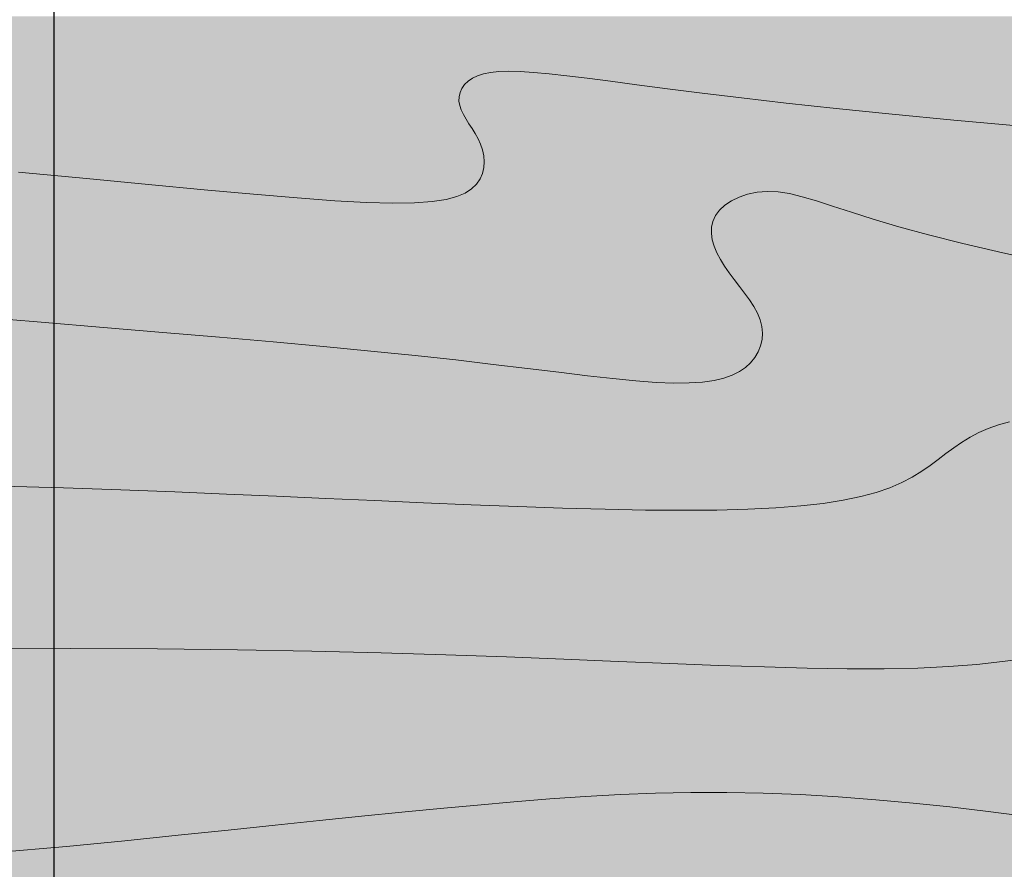
# Model space of a CAD drawing. Units: inches. Extents: x 2549 to 3108, y 1683 to 2362.
# Tile 12 of 30: x 2734 to 2749, y 2028 to 2041. Entities that reach past the tile are written whole.
import ezdxf

# ---------------------------------------------------------------- set-up
doc = ezdxf.new("R2010")
doc.units = ezdxf.units.IN
for name, color, linetype, lineweight in [('A-ANNO-DIMS', 2, 'Continuous', 18), ('A-FURN', 8, 'Continuous', 18), ('A-FURN-PATT', 9, 'Continuous', 13)]:
    doc.layers.add(name, color=color, linetype=linetype, lineweight=lineweight)
doc.layers.add('C-PKNG-VEHI-PATT', color=251, linetype='Continuous', lineweight=13, true_color=0x636466)
doc.layers.add('C-PVMT-PATT', color=9, linetype='Continuous', lineweight=13, true_color=0xc7c8ca)
doc.styles.get("Standard").update_dxf_attribs({"font": 'arial.ttf'})
doc.dimstyles.get("Standard").update_dxf_attribs({"dimtxt": 0.18, "dimasz": 0.18, "dimexe": 0.18, "dimexo": 0.0625, "dimgap": 0.09, "dimtad": 0, "dimtih": 1, "dimtoh": 1, "dimdec": 4, "dimzin": 0, "dimdsep": 46, "dimtxsty": 'Standard', "dimcen": 0.09, "dimadec": 0, "dimazin": 0, "dimtfac": 1, "dimtdec": 4, "dimtofl": 0, "dimtmove": 0, "dimatfit": 3, "dimfxl": 1, "dimtolj": 1, "dimtzin": 0, "dimarcsym": 0})

# ---------------------------------------------------------------- blocks, each defined once
blk = doc.blocks.new('Dining Set - 36 x 72 in.')
for points in [[(-3.6035, 13.63021), (-1.6954, 13.45508), (0.0365, 13.29166), (1.5945, 13.14388), (2.9811, 13.01562), (4.1988, 12.9108), (5.25, 12.83333), (6.1393, 12.78613), (6.8802, 12.76823), (7.4883, 12.77767), (7.9792, 12.8125), (8.3685, 12.87077), (8.6719, 12.95052), (8.9049, 13.0498), (9.0833, 13.16666), (9.2205, 13.29899), (9.3216, 13.44401), (9.3895, 13.59879), (9.4271, 13.76041), (9.4373, 13.92594), (9.4232, 14.09245), (9.3875, 14.257), (9.3333, 14.41666), (9.2638, 14.56917), (9.1836, 14.71484), (9.0975, 14.85465), (9.0104, 14.98958), (8.9272, 15.1206), (8.8529, 15.2487), (8.7922, 15.37483), (8.75, 15.5), (8.7305, 15.62467), (8.7344, 15.74739), (8.7617, 15.86621), (8.8125, 15.97916), (8.8867, 16.08431), (8.9844, 16.17968), (9.1055, 16.26334), (9.25, 16.33333), (9.4189, 16.38802), (9.6172, 16.42708), (9.8506, 16.45052), (10.125, 16.45833), (10.4463, 16.45052), (10.8203, 16.42708), (11.2529, 16.38802), (11.75, 16.33333), (12.3184, 16.26318), (12.9694, 16.17838), (13.7151, 16.07991), (14.5677, 15.96875), (15.5395, 15.84586), (16.6426, 15.71224), (17.8893, 15.56884), (19.2917, 15.41666), (20.859, 15.25667), (22.5879, 15.08984), (24.4721, 14.91715)], [(-4.7917, 9.58333), (-2.9698, 9.43082), (-1.2246, 9.28515), (0.4415, 9.14534), (2.026, 9.01041), (3.5266, 8.87939), (4.9408, 8.7513), (6.266, 8.62516), (7.5, 8.5), (8.6411, 8.37549), (9.6914, 8.2539), (10.6538, 8.13818), (11.5312, 8.03125), (12.3267, 7.93603), (13.043, 7.85547), (13.6831, 7.79248), (14.25, 7.75), (14.7471, 7.7303), (15.1797, 7.73307), (15.5537, 7.75732), (15.875, 7.80208), (16.1494, 7.86637), (16.3828, 7.94922), (16.5811, 8.04964), (16.75, 8.16666), (16.8944, 8.29915), (17.0143, 8.44531), (17.1089, 8.60319), (17.1771, 8.77083), (17.218, 8.94629), (17.2305, 9.1276), (17.2137, 9.31282), (17.1667, 9.5), (17.0895, 9.6875), (16.987, 9.875), (16.8649, 10.0625), (16.7292, 10.25), (16.5856, 10.4375), (16.4401, 10.625), (16.2985, 10.8125), (16.1667, 11), (16.05, 11.18733), (15.9518, 11.3737), (15.8752, 11.5581), (15.8229, 11.73958), (15.798, 11.91715), (15.8034, 12.08984), (15.842, 12.25667), (15.9167, 12.41666), (16.0295, 12.56836), (16.1784, 12.70833), (16.3605, 12.83268), (16.5729, 12.9375), (16.8127, 13.01888), (17.0768, 13.07291), (17.3625, 13.0957), (17.6667, 13.08333), (17.9894, 13.03312), (18.3418, 12.94726), (18.7382, 12.82918), (19.1927, 12.68229), (19.7195, 12.51001), (20.3327, 12.31575), (21.0465, 12.10294), (21.875, 11.875), (22.8357, 11.63354), (23.959, 11.37304), (25.2786, 11.08618)], [(-4.0586, 4.83984), (-2.3429, 4.79215), (-0.7396, 4.73958), (0.7739, 4.6831), (2.22, 4.6237), (3.6213, 4.56233), (5, 4.5), (6.373, 4.43782), (7.7344, 4.3776), (9.0723, 4.32129), (10.375, 4.27083), (11.6309, 4.22819), (12.8281, 4.19531), (13.9551, 4.17415), (15, 4.16666), (15.954, 4.17448), (16.819, 4.19791), (17.6001, 4.23698), (18.3021, 4.29166), (18.9299, 4.36198), (19.4883, 4.44791), (19.9823, 4.54948), (20.4167, 4.66666), (20.7969, 4.79899), (21.1302, 4.94401), (21.4245, 5.09879), (21.6875, 5.26041), (21.9271, 5.42594), (22.1511, 5.59245), (22.3672, 5.757), (22.5834, 5.91666), (22.8065, 6.06868), (23.0404, 6.21093), (23.2879, 6.34147), (23.5521, 6.45833), (23.8358, 6.55957), (24.142, 6.64323)], [(-4.75, 0.29166), (-2.134, 0.29793), (0.2878, 0.28711), (2.5317, 0.26163), (4.6146, 0.22396), (6.5529, 0.17651), (8.3633, 0.12174), (10.0623, 0.06209), (11.6667, 0), (13.1899, -0.06201), (14.6341, -0.1211), (15.9982, -0.17432), (17.2813, -0.21875), (18.4823, -0.25147), (19.6003, -0.26953), (20.6343, -0.27002), (21.5834, -0.25), (22.4481, -0.20768), (23.2357, -0.14584), (23.9549, -0.06836), (24.6146, 0.02083)], [(-4.2363, -5.41016), (-2.2629, -5.24333), (-0.625, -5.08334), (0.8708, -4.93099), (2.2715, -4.78646), (3.5872, -4.64974), (4.8281, -4.52084), (6.0046, -4.39974), (7.127, -4.28646), (8.2053, -4.18099), (9.25, -4.08334), (10.2705, -3.99382), (11.2734, -3.91407), (12.2647, -3.84603), (13.25, -3.79167), (14.2354, -3.75293), (15.2266, -3.73177), (16.2295, -3.73015), (17.25, -3.75), (18.2912, -3.79248), (19.3451, -3.85547), (20.4009, -3.93604), (21.4479, -4.03125), (22.4754, -4.13819), (23.4727, -4.25391), (24.4289, -4.37549)]]:
    blk.add_lwpolyline(points)
blk = doc.blocks.new('*D43')
at = {"layer": 'A-ANNO-DIMS', "color": 0, "lineweight": -2, "transparency": 16777216}
for p, q in [((2734.643, 2080.461), (2734.643, 1683.444)), ((2806.643, 2080.461), (2806.643, 1683.444)), ((2734.823, 1683.624), (2770.425, 1683.624)), ((2806.463, 1683.624), (2770.86, 1683.624))]:
    blk.add_line(p, q, dxfattribs=at)
at = {"layer": 'A-ANNO-DIMS', "color": 0, "transparency": 16777216}
for points in [[(2734.823, 1683.654), (2734.823, 1683.594), (2734.643, 1683.624)], [(2806.463, 1683.654), (2806.463, 1683.594), (2806.643, 1683.624)]]:
    blk.add_solid(points, dxfattribs=at)
at = {"layer": 'Defpoints', "color": 0, "transparency": 16777216}
for p in [(2734.643, 2080.524), (2806.643, 2080.524), (2806.643, 1683.624)]:
    blk.add_point(p, dxfattribs=at)
at = {"layer": 'A-ANNO-DIMS', "color": 0, "transparency": 16777216, "insert": (2770.643, 1683.624), "char_height": 0.18, "attachment_point": 5}
blk.add_mtext('\\A1;72', dxfattribs=at)
blk = doc.blocks.new('*D44')
at = {"layer": 'A-ANNO-DIMS', "color": 0, "lineweight": -2, "transparency": 16777216}
for p, q in [((2662.643, 2040.993), (2662.643, 1683.444)), ((2806.643, 2016.129), (2806.643, 1683.444)), ((2662.823, 1683.624), (2734.363, 1683.624)), ((2806.463, 1683.624), (2734.923, 1683.624))]:
    blk.add_line(p, q, dxfattribs=at)
at = {"layer": 'A-ANNO-DIMS', "color": 0, "transparency": 16777216}
for points in [[(2662.823, 1683.654), (2662.823, 1683.594), (2662.643, 1683.624)], [(2806.463, 1683.654), (2806.463, 1683.594), (2806.643, 1683.624)]]:
    blk.add_solid(points, dxfattribs=at)
at = {"layer": 'Defpoints', "color": 0, "transparency": 16777216}
for p in [(2662.643, 2041.056), (2806.643, 2016.191), (2806.643, 1683.624)]:
    blk.add_point(p, dxfattribs=at)
at = {"layer": 'A-ANNO-DIMS', "color": 0, "transparency": 16777216, "insert": (2734.643, 1683.624), "char_height": 0.18, "attachment_point": 5}
blk.add_mtext('\\A1;144', dxfattribs=at)
blk = doc.blocks.new('*D59')
at = {"layer": 'A-ANNO-DIMS', "color": 0, "lineweight": -2, "transparency": 16777216}
for p, q in [((2680.978, 1761.586), (2680.978, 2362.323)), ((2786.158, 1761.586), (2786.158, 2362.323)), ((2681.158, 2362.143), (2733.112, 2362.143)), ((2785.978, 2362.143), (2734.023, 2362.143))]:
    blk.add_line(p, q, dxfattribs=at)
at = {"layer": 'A-ANNO-DIMS', "color": 0, "transparency": 16777216}
for points in [[(2681.158, 2362.173), (2681.158, 2362.113), (2680.978, 2362.143)], [(2785.978, 2362.173), (2785.978, 2362.113), (2786.158, 2362.143)]]:
    blk.add_solid(points, dxfattribs=at)
at = {"layer": 'Defpoints', "color": 0, "transparency": 16777216}
for p in [(2786.158, 2362.143), (2680.978, 1761.524), (2786.158, 1761.524)]:
    blk.add_point(p, dxfattribs=at)
at = {"layer": 'A-ANNO-DIMS', "color": 0, "transparency": 16777216, "insert": (2733.568, 2362.143), "char_height": 0.18, "attachment_point": 5}
blk.add_mtext('\\A1;105.18', dxfattribs=at)

msp = doc.modelspace()

# ---------------------------------------------------------------- hatches: boundary and pattern name
at = {"layer": 'A-FURN-PATT'}
h = msp.add_hatch(color=256, dxfattribs=at)
h.dxf.hatch_style = 1
h.paths.add_polyline_path([(2744.8667, 2037.254), (2744.7754, 2037.3839), (2744.7125, 2037.4849), (2744.6595, 2037.5854), (2744.5963, 2037.7375), (2744.5695, 2037.9287), (2744.6003, 2038.0617), (2744.6406, 2038.148), (2744.7014, 2038.2298), (2744.7817, 2038.3053), (2744.8799, 2038.3724), (2744.9945, 2038.4289), (2745.1238, 2038.4728), (2745.2663, 2038.5019), (2745.4204, 2038.5142), (2745.5844, 2038.5076), (2745.7585, 2038.4805), (2745.9486, 2038.4342), (2746.1624, 2038.3705), (2746.4075, 2038.2913), (2746.6917, 2038.1983), (2747.0224, 2038.0936), (2747.4074, 2037.9788), (2747.8543, 2037.8558), (2748.3724, 2037.7256), (2748.9783, 2037.5851), (2749.69, 2037.4304), (2750.5258, 2037.2575), (2751.5038, 2037.0624), (2752.6422, 2036.8414), (2753.9591, 2036.5902), (2755.4728, 2036.3051), (2755.4728, 2039.002), (2754.0892, 2039.103), (2752.7721, 2039.2035), (2751.5251, 2039.303), (2750.3516, 2039.4009), (2749.255, 2039.4967), (2748.2388, 2039.5898), (2747.3063, 2039.6798), (2746.4609, 2039.7661), (2745.7045, 2039.8482), (2745.0321, 2039.9255), (2744.4371, 2039.9976), (2743.9129, 2040.0639), (2743.4531, 2040.1238), (2743.0509, 2040.1769), (2742.6998, 2040.2227), (2742.3932, 2040.2605), (2742.1251, 2040.29), (2741.8917, 2040.3111), (2741.69, 2040.3237), (2741.5167, 2040.3279), (2741.3687, 2040.3237), (2741.2428, 2040.3111), (2741.1359, 2040.29), (2741.0448, 2040.2605), (2740.9668, 2040.2227), (2740.9015, 2040.1776), (2740.8488, 2040.1262), (2740.8088, 2040.0695), (2740.7814, 2040.0085), (2740.7667, 2039.9445), (2740.7646, 2039.8783), (2740.7751, 2039.811), (2740.7978, 2039.7435), (2740.8306, 2039.6755), (2740.8707, 2039.6064), (2740.9155, 2039.5357), (2740.996, 2039.4111), (2741.0771, 2039.2637), (2741.1346, 2039.0945), (2741.1499, 2038.9139), (2741.1092, 2038.7391), (2741.0289, 2038.6239), (2740.9549, 2038.5525), (2740.8586, 2038.4895), (2740.733, 2038.4359), (2740.5693, 2038.3929), (2740.3593, 2038.3615), (2740.0946, 2038.3427), (2739.7666, 2038.3376), (2739.367, 2038.3473), (2738.8873, 2038.3727), (2738.3203, 2038.4145), (2737.6635, 2038.471), (2736.9156, 2038.5402), (2736.0753, 2038.6199), (2735.1412, 2038.7081), (2734.112, 2038.8025), (2732.9864, 2038.9012), (2731.7632, 2039.002), (2730.4376, 2039.1026), (2728.9922, 2039.2), (2727.4062, 2039.2911), (2725.6588, 2039.3728), (2723.7291, 2039.4418), (2721.5964, 2039.495), (2719.2397, 2039.5292), (2716.6384, 2039.5413), (2716.6384, 2036.8445), (2720.4266, 2036.9215), (2723.5572, 2036.9548), (2726.1183, 2036.9512), (2728.1983, 2036.9175), (2729.8853, 2036.8608), (2731.2677, 2036.7876), (2732.4336, 2036.705), (2733.4711, 2036.6198), (2734.4538, 2036.5375), (2735.3951, 2036.4589), (2736.2938, 2036.3835), (2737.1484, 2036.3108), (2737.9578, 2036.2401), (2738.7205, 2036.171), (2739.4353, 2036.103), (2740.1009, 2036.0355), (2740.7163, 2035.9683), (2741.2828, 2035.9027), (2741.8019, 2035.8403), (2742.2752, 2035.7826), (2742.7042, 2035.7313), (2743.0906, 2035.6878), (2743.4358, 2035.6539), (2743.7416, 2035.6309), (2744.0097, 2035.6203), (2744.243, 2035.6218), (2744.4448, 2035.6349), (2744.6181, 2035.659), (2744.7661, 2035.6937), (2744.892, 2035.7384), (2744.9989, 2035.7926), (2745.09, 2035.8557), (2745.1679, 2035.9271), (2745.2326, 2036.006), (2745.2836, 2036.0911), (2745.3204, 2036.1815), (2745.3424, 2036.2762), (2745.3492, 2036.374), (2745.3401, 2036.4739), (2745.3148, 2036.5748), (2745.2731, 2036.676), (2745.2178, 2036.7771), (2745.152, 2036.8782), (2745.0788, 2036.9794), (2745.0013, 2037.0805)])
h.paths.add_polyline_path([(2755.4728, 2036.3051), (2753.9591, 2036.5902), (2752.6422, 2036.8414), (2751.5038, 2037.0624), (2750.5258, 2037.2575), (2749.69, 2037.4304), (2748.9783, 2037.5851), (2748.3724, 2037.7256), (2747.8543, 2037.8558), (2747.4074, 2037.9788), (2747.0224, 2038.0936), (2746.6917, 2038.1983), (2746.4075, 2038.2913), (2746.1624, 2038.3705), (2745.9486, 2038.4342), (2745.7585, 2038.4805), (2745.5844, 2038.5076), (2745.4204, 2038.5142), (2745.2663, 2038.5019), (2745.1238, 2038.4728), (2744.9945, 2038.4289), (2744.8799, 2038.3724), (2744.7817, 2038.3053), (2744.7014, 2038.2298), (2744.6406, 2038.148), (2744.6003, 2038.0617), (2744.5794, 2037.9717), (2744.5765, 2037.8786), (2744.59, 2037.7828), (2744.6182, 2037.6849), (2744.6595, 2037.5854), (2744.7125, 2037.4849), (2744.7754, 2037.3839), (2744.8465, 2037.2827), (2744.9229, 2037.1816), (2745.0013, 2037.0805), (2745.1278, 2036.9154), (2745.2178, 2036.7771), (2745.2731, 2036.676), (2745.3148, 2036.5748), (2745.3401, 2036.4739), (2745.3492, 2036.374), (2745.3424, 2036.2762), (2745.3204, 2036.1815), (2745.2836, 2036.0911), (2745.2326, 2036.006), (2745.1679, 2035.9271), (2745.09, 2035.8557), (2744.9989, 2035.7926), (2744.892, 2035.7384), (2744.7661, 2035.6937), (2744.6181, 2035.659), (2744.4448, 2035.6349), (2744.243, 2035.6218), (2744.0097, 2035.6203), (2743.7416, 2035.6309), (2743.4358, 2035.6539), (2743.0906, 2035.6878), (2742.7042, 2035.7313), (2742.2752, 2035.7826), (2741.8019, 2035.8403), (2741.2828, 2035.9027), (2740.7163, 2035.9683), (2740.1009, 2036.0355), (2739.4353, 2036.103), (2738.7205, 2036.171), (2737.9578, 2036.2401), (2737.1484, 2036.3108), (2736.2938, 2036.3835), (2735.3951, 2036.4589), (2734.4538, 2036.5375), (2733.4711, 2036.6198), (2732.4336, 2036.705), (2731.2677, 2036.7876), (2729.8853, 2036.8608), (2728.1983, 2036.9175), (2726.1183, 2036.9512), (2723.5572, 2036.9548), (2720.4266, 2036.9215), (2716.6384, 2036.8445), (2716.6384, 2034.4174), (2719.4886, 2034.3283), (2721.9949, 2034.2608), (2724.1925, 2034.2112), (2726.1167, 2034.1758), (2727.8028, 2034.1509), (2729.2861, 2034.1329), (2730.602, 2034.1181), (2731.7856, 2034.1027), (2732.8685, 2034.0839), (2733.8666, 2034.0613), (2734.7919, 2034.0356), (2735.6567, 2034.0072), (2736.473, 2033.9768), (2737.253, 2033.9447), (2738.0088, 2033.9116), (2738.7525, 2033.878), (2739.493, 2033.8445), (2740.2273, 2033.812), (2740.9489, 2033.7816), (2741.6515, 2033.7544), (2742.3289, 2033.7314), (2742.9747, 2033.7137), (2743.5825, 2033.7022), (2744.1461, 2033.6982), (2744.6607, 2033.7024), (2745.1272, 2033.7151), (2745.5485, 2033.7361), (2745.9272, 2033.7656), (2746.2658, 2033.8036), (2746.567, 2033.8499), (2746.8334, 2033.9047), (2747.0677, 2033.9679), (2747.2728, 2034.0393), (2747.4525, 2034.1175), (2747.6113, 2034.201), (2747.7531, 2034.2881), (2747.8824, 2034.3774), (2748.0032, 2034.4672), (2748.1197, 2034.556), (2748.2363, 2034.6421), (2748.3567, 2034.7241), (2748.4828, 2034.8008), (2748.6163, 2034.8712), (2748.7588, 2034.9343), (2748.9118, 2034.9889), (2749.077, 2035.034), (2749.2558, 2035.0686), (2749.4499, 2035.0916), (2749.6603, 2035.1022), (2749.8861, 2035.1007), (2750.1254, 2035.0876), (2750.3769, 2035.0635), (2750.639, 2035.0288), (2750.91, 2034.9841), (2751.1884, 2034.93), (2751.4725, 2034.8668), (2751.7642, 2034.7949), (2752.0786, 2034.7123), (2752.4341, 2034.6172), (2752.849, 2034.5073), (2753.3419, 2034.3805), (2753.9313, 2034.2348), (2754.6354, 2034.068), (2755.4728, 2033.878)])
h.paths.add_polyline_path([(2755.4728, 2033.878), (2754.6354, 2034.068), (2753.9313, 2034.2348), (2753.3419, 2034.3805), (2752.849, 2034.5073), (2752.4341, 2034.6172), (2752.0786, 2034.7123), (2751.7642, 2034.7949), (2751.4725, 2034.8668), (2751.1884, 2034.93), (2750.91, 2034.9841), (2750.639, 2035.0288), (2750.3769, 2035.0635), (2750.1254, 2035.0876), (2749.8861, 2035.1007), (2749.6603, 2035.1022), (2749.4499, 2035.0916), (2749.2558, 2035.0686), (2749.077, 2035.034), (2748.9118, 2034.9889), (2748.7588, 2034.9343), (2748.6163, 2034.8712), (2748.4828, 2034.8008), (2748.3567, 2034.7241), (2748.2363, 2034.6421), (2748.1197, 2034.556), (2748.0032, 2034.4672), (2747.8824, 2034.3774), (2747.7531, 2034.2881), (2747.6113, 2034.201), (2747.4525, 2034.1175), (2747.2728, 2034.0393), (2747.0677, 2033.9679), (2746.8334, 2033.9047), (2746.567, 2033.8499), (2746.2658, 2033.8036), (2745.9272, 2033.7656), (2745.5485, 2033.7361), (2745.1272, 2033.7151), (2744.6607, 2033.7024), (2744.1461, 2033.6982), (2743.5825, 2033.7022), (2742.9747, 2033.7137), (2742.3289, 2033.7314), (2741.6515, 2033.7544), (2740.9489, 2033.7816), (2740.2273, 2033.812), (2739.493, 2033.8445), (2738.7525, 2033.878), (2738.0088, 2033.9116), (2737.253, 2033.9447), (2736.473, 2033.9768), (2735.6567, 2034.0072), (2734.7919, 2034.0356), (2733.8666, 2034.0613), (2732.8685, 2034.0839), (2731.7856, 2034.1027), (2730.602, 2034.1181), (2729.2861, 2034.1329), (2727.8028, 2034.1509), (2726.1167, 2034.1758), (2724.1925, 2034.2112), (2721.9949, 2034.2608), (2719.4886, 2034.3283), (2716.6384, 2034.4174), (2716.6384, 2030.9115), (2719.4477, 2031.0954), (2722.0216, 2031.2447), (2724.3773, 2031.363), (2726.5324, 2031.4537), (2728.5042, 2031.5201), (2730.3101, 2031.5657), (2731.9674, 2031.5939), (2733.4936, 2031.6082), (2734.9046, 2031.6115), (2736.2109, 2031.6057), (2737.4211, 2031.592), (2738.5446, 2031.5716), (2739.59, 2031.5461), (2740.5665, 2031.5165), (2741.4829, 2031.4843), (2742.3482, 2031.4509), (2743.1698, 2031.4174), (2743.9488, 2031.3855), (2744.6845, 2031.3568), (2745.3766, 2031.3329), (2746.0244, 2031.3152), (2746.6274, 2031.3055), (2747.1851, 2031.3052), (2747.697, 2031.316), (2748.1634, 2031.3388), (2748.5882, 2031.3722), (2748.9761, 2031.414), (2749.3319, 2031.4621), (2749.6603, 2031.5144), (2749.9661, 2031.5688), (2750.254, 2031.6233), (2750.5287, 2031.6756), (2750.7946, 2031.7239), (2751.0553, 2031.7669), (2751.314, 2031.8036), (2751.5737, 2031.8329), (2751.8375, 2031.8538), (2752.1088, 2031.8652), (2752.3906, 2031.8661), (2752.6861, 2031.8554), (2752.9965, 2031.8326), (2753.315, 2031.7999), (2753.633, 2031.7598), (2753.9418, 2031.7149), (2754.2327, 2031.6679), (2754.497, 2031.6215), (2754.7259, 2031.5782), (2754.911, 2031.5407), (2755.0467, 2031.5111), (2755.141, 2031.4888), (2755.2053, 2031.4728), (2755.2509, 2031.4621), (2755.2891, 2031.4556), (2755.3313, 2031.4523), (2755.3888, 2031.451), (2755.4728, 2031.4509)])
h.paths.add_polyline_path([(2743.9488, 2031.3855), (2743.1698, 2031.4174), (2742.3482, 2031.4509), (2741.4829, 2031.4843), (2740.5665, 2031.5165), (2739.59, 2031.5461), (2738.5446, 2031.5716), (2737.4211, 2031.592), (2736.2109, 2031.6057), (2734.9046, 2031.6115), (2733.4936, 2031.6082), (2731.9674, 2031.5939), (2730.3101, 2031.5657), (2728.5042, 2031.5201), (2726.5324, 2031.4537), (2724.3773, 2031.363), (2722.0216, 2031.2447), (2719.4477, 2031.0954), (2716.6384, 2030.9115), (2716.6384, 2027.945), (2721.3933, 2028.046), (2725.223, 2028.1465), (2728.2515, 2028.246), (2730.603, 2028.3439), (2732.4013, 2028.4397), (2733.7707, 2028.5328), (2734.8351, 2028.6228), (2735.7185, 2028.7091), (2736.5253, 2028.7912), (2737.2808, 2028.8692), (2737.9904, 2028.9429), (2738.6597, 2029.0125), (2739.2943, 2029.0778), (2739.8997, 2029.1389), (2740.4813, 2029.1958), (2741.0448, 2029.2484), (2741.5952, 2029.2967), (2742.1361, 2029.3397), (2742.6708, 2029.3764), (2743.2022, 2029.4058), (2743.7337, 2029.4266), (2744.2683, 2029.4381), (2744.8093, 2029.4389), (2745.3597, 2029.4282), (2745.9213, 2029.4053), (2746.4897, 2029.3713), (2747.0592, 2029.3279), (2747.6239, 2029.2765), (2748.1781, 2029.2189), (2748.716, 2029.1564), (2749.2317, 2029.0909), (2749.7196, 2029.0237), (2750.1754, 2028.9563), (2750.602, 2028.8892), (2751.0039, 2028.8226), (2751.3854, 2028.7568), (2751.7512, 2028.6921), (2752.1057, 2028.6287), (2752.4532, 2028.5668), (2752.7985, 2028.5068), (2753.1447, 2028.4496), (2753.4913, 2028.399), (2753.8363, 2028.3595), (2754.1778, 2028.3355), (2754.514, 2028.3315), (2754.8432, 2028.352), (2755.1634, 2028.4014), (2755.4728, 2028.4843), (2755.4728, 2031.4509), (2755.3151, 2031.4512), (2755.2429, 2031.4634), (2755.141, 2031.4888), (2755.0467, 2031.5111), (2754.911, 2031.5407), (2754.7259, 2031.5782), (2754.497, 2031.6215), (2754.2327, 2031.6679), (2753.9418, 2031.7149), (2753.633, 2031.7598), (2753.315, 2031.7999), (2752.9965, 2031.8326), (2752.6861, 2031.8554), (2752.3906, 2031.8661), (2752.1088, 2031.8652), (2751.8375, 2031.8538), (2751.5737, 2031.8329), (2751.314, 2031.8036), (2751.0553, 2031.7669), (2750.7946, 2031.7239), (2750.5287, 2031.6756), (2750.254, 2031.6233), (2749.9661, 2031.5688), (2749.6603, 2031.5144), (2749.3319, 2031.4621), (2748.9761, 2031.414), (2748.5882, 2031.3722), (2748.1634, 2031.3388), (2747.697, 2031.316), (2747.1851, 2031.3052), (2746.6274, 2031.3055), (2746.0244, 2031.3152), (2745.3766, 2031.3329), (2744.6845, 2031.3568)])
h.paths.add_polyline_path([(2755.4728, 2028.4843), (2755.1634, 2028.4014), (2754.8432, 2028.352), (2754.514, 2028.3315), (2754.1778, 2028.3355), (2753.8363, 2028.3595), (2753.4913, 2028.399), (2753.1447, 2028.4496), (2752.7985, 2028.5068), (2752.4532, 2028.5668), (2752.1057, 2028.6287), (2751.7512, 2028.6921), (2751.3854, 2028.7568), (2751.0039, 2028.8226), (2750.602, 2028.8892), (2750.1754, 2028.9563), (2749.7196, 2029.0237), (2749.2317, 2029.0909), (2748.716, 2029.1564), (2748.1781, 2029.2189), (2747.6239, 2029.2765), (2747.0592, 2029.3279), (2746.4897, 2029.3713), (2745.9213, 2029.4053), (2745.3597, 2029.4282), (2744.8093, 2029.4389), (2744.2683, 2029.4381), (2743.7337, 2029.4266), (2743.2022, 2029.4058), (2742.6708, 2029.3764), (2742.1361, 2029.3397), (2741.5952, 2029.2967), (2741.0448, 2029.2484), (2740.4813, 2029.1958), (2739.8997, 2029.1389), (2739.2943, 2029.0778), (2738.6597, 2029.0125), (2737.9904, 2028.9429), (2737.2808, 2028.8692), (2736.5253, 2028.7912), (2735.7185, 2028.7091), (2734.8351, 2028.6228), (2733.7707, 2028.5328), (2732.4013, 2028.4397), (2730.603, 2028.3439), (2728.2515, 2028.246), (2725.223, 2028.1465), (2721.3933, 2028.046), (2716.6384, 2027.945), (2716.6384, 2023.63), (2719.8271, 2023.719), (2722.5536, 2023.7853), (2724.8739, 2023.8315), (2726.8443, 2023.8604), (2728.5207, 2023.8745), (2729.9593, 2023.8765), (2731.2162, 2023.8691), (2732.3475, 2023.8548), (2733.4006, 2023.8359), (2734.3887, 2023.8133), (2735.3162, 2023.7876), (2736.1877, 2023.7593), (2737.0074, 2023.7288), (2737.7801, 2023.6968), (2738.5101, 2023.6637), (2739.2019, 2023.63), (2739.8611, 2023.5965), (2740.4973, 2023.5644), (2741.1215, 2023.5348), (2741.7443, 2023.5092), (2742.3766, 2023.4889), (2743.0291, 2023.4752), (2743.7127, 2023.4693), (2744.4383, 2023.4727), (2745.2212, 2023.4875), (2746.096, 2023.5194), (2747.1021, 2023.575), (2748.2785, 2023.6609), (2749.6645, 2023.7837), (2751.2994, 2023.9499), (2753.2224, 2024.1662), (2755.4728, 2024.4391)])
h.paths.add_polyline_path([(2755.4728, 2026.3269), (2754.9554, 2026.3329), (2754.418, 2026.3497), (2753.8658, 2026.3755), (2753.3041, 2026.4083), (2752.7382, 2026.4465), (2752.1734, 2026.4881), (2751.6149, 2026.5312), (2751.068, 2026.5741), (2750.5357, 2026.6151), (2750.0124, 2026.6538), (2749.4902, 2026.6898), (2748.9611, 2026.723), (2748.4173, 2026.753), (2747.8508, 2026.7795), (2747.2537, 2026.8024), (2746.6182, 2026.8213), (2745.9367, 2026.8359), (2745.2024, 2026.8452), (2744.4091, 2026.8482), (2743.5505, 2026.8438), (2742.6204, 2026.8309), (2741.6122, 2026.8087), (2740.5198, 2026.7758), (2739.3368, 2026.7314), (2738.0388, 2026.6748), (2736.5297, 2026.6071), (2734.695, 2026.5299), (2732.4205, 2026.4449), (2729.5919, 2026.3535), (2726.0949, 2026.2573), (2721.8152, 2026.1581), (2716.6384, 2026.0572), (2716.6384, 2023.63), (2719.8271, 2023.719), (2722.5536, 2023.7853), (2724.8739, 2023.8315), (2726.8443, 2023.8604), (2728.5207, 2023.8745), (2729.9593, 2023.8765), (2731.2162, 2023.8691), (2732.3475, 2023.8548), (2733.4006, 2023.8359), (2734.3887, 2023.8133), (2735.3162, 2023.7876), (2736.1877, 2023.7593), (2737.0074, 2023.7288), (2737.7801, 2023.6968), (2738.5101, 2023.6637), (2739.2019, 2023.63), (2739.8611, 2023.5965), (2740.4973, 2023.5644), (2741.1215, 2023.5348), (2741.7443, 2023.5092), (2742.3766, 2023.4889), (2743.0291, 2023.4752), (2743.7127, 2023.4693), (2744.4383, 2023.4727), (2745.2212, 2023.4875), (2746.096, 2023.5194), (2747.1021, 2023.575), (2748.2785, 2023.6609), (2749.6645, 2023.7837), (2751.2994, 2023.9499), (2753.2224, 2024.1662), (2755.4728, 2024.4391)], flags=17)
h.paths.add_polyline_path([(2740.4973, 2023.5644), (2739.8611, 2023.5965), (2739.2019, 2023.63), (2738.5101, 2023.6637), (2737.7801, 2023.6968), (2737.0074, 2023.7288), (2736.1877, 2023.7593), (2735.3162, 2023.7876), (2734.3887, 2023.8133), (2733.4006, 2023.8359), (2732.3475, 2023.8548), (2731.2162, 2023.8691), (2729.9593, 2023.8765), (2728.5207, 2023.8745), (2726.8443, 2023.8604), (2724.8739, 2023.8315), (2722.5536, 2023.7853), (2719.8271, 2023.719), (2716.6384, 2023.63), (2716.6384, 2021.7423), (2755.4728, 2021.7423), (2755.4728, 2024.4391), (2753.2224, 2024.1662), (2751.2994, 2023.9499), (2749.6645, 2023.7837), (2748.2785, 2023.6609), (2747.1021, 2023.575), (2746.096, 2023.5194), (2745.2212, 2023.4875), (2744.4383, 2023.4727), (2743.7127, 2023.4693), (2743.0291, 2023.4752), (2742.3766, 2023.4889), (2741.7443, 2023.5092), (2741.1215, 2023.5348)])
h.paths.add_polyline_path([(2741.1359, 2040.29), (2741.2428, 2040.3111), (2741.3687, 2040.3237), (2741.5167, 2040.3279), (2741.69, 2040.3237), (2741.8917, 2040.3111), (2742.1251, 2040.29), (2742.3932, 2040.2605), (2742.6998, 2040.2227), (2743.0509, 2040.1769), (2743.4531, 2040.1238), (2743.9129, 2040.0639), (2744.4371, 2039.9976), (2745.0321, 2039.9255), (2745.7045, 2039.8482), (2746.4609, 2039.7661), (2747.3063, 2039.6798), (2748.2388, 2039.5898), (2749.255, 2039.4967), (2750.3516, 2039.4009), (2751.5251, 2039.303), (2752.7721, 2039.2035), (2754.0892, 2039.103), (2755.4728, 2039.002), (2755.4728, 2041.1594), (2716.6384, 2041.1594), (2716.6384, 2039.5413), (2719.2397, 2039.5292), (2721.5964, 2039.495), (2723.7291, 2039.4418), (2725.6588, 2039.3728), (2727.4062, 2039.2911), (2728.9922, 2039.2), (2730.4376, 2039.1026), (2731.7632, 2039.002), (2732.9864, 2038.9012), (2734.112, 2038.8025), (2735.1412, 2038.7081), (2736.0753, 2038.6199), (2736.9156, 2038.5402), (2737.6635, 2038.471), (2738.3203, 2038.4145), (2738.8873, 2038.3727), (2739.367, 2038.3473), (2739.7666, 2038.3376), (2740.0946, 2038.3427), (2740.3593, 2038.3615), (2740.5693, 2038.3929), (2740.733, 2038.4359), (2740.8586, 2038.4895), (2740.9549, 2038.5525), (2741.0289, 2038.6239), (2741.0834, 2038.7021), (2741.12, 2038.7856), (2741.1403, 2038.8728), (2741.1458, 2038.962), (2741.1382, 2039.0518), (2741.1189, 2039.1406), (2741.0897, 2039.2267), (2741.0522, 2039.309), (2741.0089, 2039.3875), (2740.9625, 2039.4629), (2740.8772, 2039.5951), (2740.8072, 2039.7159), (2740.7635, 2039.8453), (2740.7677, 2039.9782), (2740.8229, 2040.1009), (2740.9289, 2040.2044), (2741.0448, 2040.2605)])
at = {"layer": 'C-PKNG-VEHI-PATT'}
h = msp.add_hatch(color=256, dxfattribs=at)
h.dxf.hatch_style = 1
edge = h.paths.add_edge_path()
edge.add_ellipse((2935.7258, 1791.964), major_axis=(-50.66, 0), ratio=0.8423039, start_angle=248.16505, end_angle=265.72258)
edge.add_line((2938.911, 1834.5507), (2925.8653, 1834.5507))
edge.add_ellipse((2929.0505, 1791.964), major_axis=(50.66, 0), ratio=0.8423039, start_angle=94.27742, end_angle=111.83495)
edge.add_line((2912.8508, 1832.3947), (2914.2044, 1822.2495))
edge.add_ellipse((2930.6538, 1783.1023), major_axis=(-49.3014, 0), ratio=0.8423039, start_angle=-85.12993, end_angle=-67.20809, ccw=False)
edge.add_line((2927.1247, 1824.5225), (2937.6516, 1824.5225))
edge.add_ellipse((2934.1225, 1783.1023), major_axis=(49.3014, 0), ratio=0.8423039, start_angle=67.20809, end_angle=85.12993, ccw=False)
edge.add_line((2950.5719, 1822.2495), (2951.9255, 1832.3947))
edge = h.paths.add_edge_path()
edge.add_ellipse((2903.4793, 1857.3351), major_axis=(-34.7979, 0), ratio=0.8423039, start_angle=180, end_angle=209.43857)
edge.add_ellipse((2961.297, 1857.3351), major_axis=(34.7979, 0), ratio=0.8423039, start_angle=150.56143, end_angle=180)
edge.add_line((2926.4991, 1857.3351), (2926.4991, 1843.7609))
edge.add_ellipse((2924.1251, 1844.3143), major_axis=(-0.2209, 3.9278), ratio=0.6038336, start_angle=89.00201, end_angle=253.65741, ccw=False)
edge.add_line((2921.7512, 1844.2222), (2921.7512, 1853.3975))
edge.add_line((2921.7512, 1853.3975), (2925.269, 1855.8484))
edge.add_ellipse((2925.4782, 1855.4931), major_axis=(0.4584, 0), ratio=0.8423039, start_angle=90, end_angle=134.48021, ccw=False)
edge.add_line((2925.4782, 1855.8792), (2926.4991, 1855.8792))
edge.add_line((2926.4991, 1855.8792), (2926.4991, 1857.3351))
edge.add_ellipse((2961.297, 1857.3351), major_axis=(34.7979, 0), ratio=0.8423039, start_angle=150.56143, end_angle=180, ccw=False)
edge.add_line((2932.3882, 1873.6501), (2932.3882, 1875.7801))
edge.add_ellipse((2932.3882, 1875.3939), major_axis=(0.4584, 0), ratio=0.8423039, start_angle=90, end_angle=127.93313)
edge.add_line((2932.1366, 1875.7167), (2928.5915, 1873.7564))
edge.add_ellipse((2899.9271, 2002.4692), major_axis=(155.4756, 0), ratio=0.84230387, start_angle=-80.743434, end_angle=-77.445067, ccw=False)
edge.add_ellipse((2949.4402, 1715.2151), major_axis=(-189.1422, 0), ratio=0.84230387, start_angle=-79.790461, end_angle=-77.555373)
edge.add_ellipse((3300.3614, 1852.5642), major_axis=(-386.1662, 0), ratio=0.84230387, start_angle=-2.863715, end_angle=2.198541)
edge.add_ellipse((2929.0505, 1792.5159), major_axis=(-55.6192, 0), ratio=0.8423039, start_angle=-85.91759, end_angle=-72.28005, ccw=False)
edge.add_line((2925.7129, 1839.2798), (2939.0634, 1839.2798))
edge.add_ellipse((2935.7258, 1792.5159), major_axis=(55.6192, 0), ratio=0.8423039, start_angle=72.28005, end_angle=85.91759, ccw=False)
edge.add_ellipse((2564.4149, 1852.5642), major_axis=(-386.1662, 0), ratio=0.84230387, start_angle=177.801459, end_angle=182.863715)
edge.add_ellipse((2915.3361, 1715.2151), major_axis=(189.1422, 0), ratio=0.84230387, start_angle=77.555373, end_angle=79.790461)
edge.add_ellipse((2964.8492, 2002.4692), major_axis=(-155.4756, 0), ratio=0.84230387, start_angle=77.445067, end_angle=80.743434, ccw=False)
edge.add_line((2936.1848, 1873.7564), (2932.6397, 1875.7167))
edge.add_ellipse((2932.3882, 1875.3939), major_axis=(0.4584, 0), ratio=0.8423039, start_angle=52.06687, end_angle=90)
edge.add_line((2932.3882, 1875.7801), (2932.3882, 1873.6501))
edge.add_ellipse((2903.4793, 1857.3351), major_axis=(-34.7979, 0), ratio=0.8423039, start_angle=180, end_angle=209.43857, ccw=False)
edge.add_line((2938.2772, 1857.3351), (2938.2772, 1855.8792))
edge.add_line((2938.2772, 1855.8792), (2939.4059, 1855.8792))
edge.add_ellipse((2939.2981, 1855.4931), major_axis=(-0.4584, 0), ratio=0.8423039, start_angle=225.51979, end_angle=270, ccw=False)
edge.add_line((2939.5903, 1855.7906), (2943.0251, 1853.3975))
edge.add_line((2943.0251, 1853.3975), (2943.0251, 1844.2222))
edge.add_ellipse((2940.6512, 1844.3143), major_axis=(0.2209, 3.9278), ratio=0.6038336, start_angle=106.34259, end_angle=270.99799, ccw=False)
edge.add_line((2938.2772, 1843.7609), (2938.2772, 1857.3351))
edge = h.paths.add_edge_path()
edge.add_ellipse((2932.3882, 1865.1973), major_axis=(91.081, 0), ratio=0.8423039, start_angle=256.401865, end_angle=283.598135, ccw=False)
edge.add_line((2914.2044, 1790.0239), (2914.2044, 1778.3622))
edge.add_ellipse((2932.3882, 1853.5356), major_axis=(91.081, 0), ratio=0.8423039, start_angle=256.401865, end_angle=283.598135)
edge.add_line((2950.5719, 1778.3622), (2950.5719, 1790.0239))
edge = h.paths.add_edge_path()
edge.add_ellipse((2948.7383, 1772.3145), major_axis=(1.8336, 0), ratio=0.8423039, start_angle=0, end_angle=90)
edge.add_line((2948.7383, 1773.859), (2916.038, 1773.859))
edge.add_ellipse((2916.038, 1772.3145), major_axis=(1.8336, 0), ratio=0.8423039, start_angle=90, end_angle=180)
edge.add_line((2914.2044, 1772.3145), (2914.2044, 1760.2558))
edge.add_line((2914.2044, 1760.2558), (2950.5719, 1760.2558))
edge.add_line((2950.5719, 1760.2558), (2950.5719, 1772.3145))
h.paths.add_polyline_path([(2748.8496, 2101.6383), (2798.148, 2101.6383), (2798.148, 2111.4248), (2748.8496, 2111.4248)], flags=9)
h.paths.add_polyline_path([(2685.2081, 2101.489), (2719.3253, 2101.489), (2719.3253, 2111.2819), (2685.2081, 2111.2819)], flags=9)
h.paths.add_polyline_path([(2814.6852, 1907.1328), (2847.8384, 1907.1328), (2847.8384, 1916.9258), (2814.6852, 1916.9258)], flags=9)
h.paths.add_polyline_path([(2814.3906, 1835.5864), (2848.0172, 1835.5864), (2848.0172, 1845.3794), (2814.3906, 1845.3794)], flags=9)
h.paths.add_polyline_path([(2800.5245, 1759.1674), (2853.7435, 1759.1674), (2853.7435, 1768.954), (2800.5245, 1768.954)], flags=9)
h.paths.add_polyline_path([(2972.4611, 1807.3305), (3015.3943, 1807.3305), (3015.3943, 1817.117), (2972.4611, 1817.117)], flags=9)
h.paths.add_polyline_path([(2902.3327, 1888.6731), (2937.9131, 1888.6731), (2937.9131, 1898.4661), (2902.3327, 1898.4661)], flags=9)
h.paths.add_polyline_path([(2712.1779, 1878.9039), (2754.1257, 1878.9039), (2754.1257, 1888.6904), (2712.1779, 1888.6904)], flags=9)
h.paths.add_polyline_path([(2614.0056, 2012.812), (2650.0251, 2012.812), (2650.0251, 2022.4371), (2614.0056, 2022.4371)], flags=9)
h.paths.add_polyline_path([(2713.3129, 2003.1645), (2747.4237, 2003.1645), (2747.4237, 2012.951), (2713.3129, 2012.951)], flags=9)
h.paths.add_polyline_path([(2950.1379, 2001.6934), (2982.2992, 2001.6934), (2982.2992, 2011.48), (2950.1379, 2011.48)], flags=9)
h.paths.add_polyline_path([(2940.864, 2238.5537), (2997.5066, 2238.5537), (2997.5066, 2248.3466), (2940.864, 2248.3466)], flags=9)
h.paths.add_polyline_path([(2821.5457, 2202.8348), (2855.663, 2202.8348), (2855.663, 2212.6278), (2821.5457, 2212.6278)], flags=9)
h.paths.add_polyline_path([(2661.8026, 2238.6249), (2718.4451, 2238.6249), (2718.4451, 2248.4179), (2661.8026, 2248.4179)], flags=9)
at = {"layer": 'C-PVMT-PATT'}
h = msp.add_hatch(color=256, dxfattribs=at)
h.dxf.hatch_style = 1
h.paths.add_polyline_path([(3067.6427, 2305.5237), (2605.6427, 2305.5237), (2605.6427, 2074.5237), (2629.6427, 2074.5237), (2629.6427, 2281.5237), (3043.6427, 2281.5237), (3043.6427, 1885.5237), (3043.6427, 1872.8745), (3031.1672, 1872.8745), (3031.1672, 1862.5731), (2995.8054, 1862.5731), (2995.8054, 1872.8745), (2983.1752, 1872.8745), (2983.1752, 1885.5237), (2881.6427, 1885.5237), (2881.6427, 1795.5237), (2751.0977, 1795.5237), (2751.0977, 1761.5237), (2786.1577, 1761.5237), (2786.1577, 1723.5237), (2881.84, 1723.5237), (2881.84, 1714.5237), (3067.6427, 1714.5237), (3067.6427, 1723.5237)])
edge = h.paths.add_edge_path(flags=16)
edge.add_ellipse((2949.4402, 1710.9683), major_axis=(-194.1014, 0), ratio=0.84230387, start_angle=-77.874034, end_angle=-76.219471, ccw=False)
edge.add_ellipse((2949.4402, 1715.2151), major_axis=(-189.1422, 0), ratio=0.84230387, start_angle=-79.790461, end_angle=-77.555373, ccw=False)
edge.add_ellipse((2899.9271, 2002.4692), major_axis=(155.4756, 0), ratio=0.84230387, start_angle=-80.743434, end_angle=-77.445067)
edge.add_line((2928.5915, 1873.7564), (2932.3882, 1875.8558))
edge.add_line((2932.3882, 1875.8558), (2936.1848, 1873.7564))
edge.add_ellipse((2964.8492, 2002.4692), major_axis=(-155.4756, 0), ratio=0.84230387, start_angle=77.445067, end_angle=80.743434)
edge.add_ellipse((2915.3361, 1715.2151), major_axis=(189.1422, 0), ratio=0.84230387, start_angle=77.555373, end_angle=79.790461, ccw=False)
edge.add_ellipse((2915.3361, 1710.9683), major_axis=(-194.1014, 0), ratio=0.84230387, start_angle=256.219471, end_angle=257.874034, ccw=False)
edge.add_ellipse((2628.2871, 1850.2612), major_axis=(-327.2532, 0), ratio=0.84230387, start_angle=182.17995, end_angle=183.650428, ccw=False)
edge.add_ellipse((2955.5637, 1861.9334), major_axis=(-0.9168, 0), ratio=0.8423039, start_angle=180, end_angle=270, ccw=False)
edge.add_line((2956.4805, 1862.3857), (2956.4805, 1846.4866))
edge.add_ellipse((2955.5637, 1846.939), major_axis=(-0.9168, 0), ratio=0.8423039, start_angle=90, end_angle=180, ccw=False)
edge.add_ellipse((-3607.0606, 1835.832), major_axis=(-6562.6242, 0), ratio=0.84230387, start_angle=179.61613322, end_angle=180.09022909, ccw=False)
edge.add_ellipse((2955.5637, 1791.0926), major_axis=(0.9168, 0), ratio=0.8423039, start_angle=0, end_angle=90, ccw=False)
edge.add_line((2956.4805, 1791.545), (2956.4805, 1775.6459))
edge.add_ellipse((2955.5637, 1776.0982), major_axis=(0.9168, 0), ratio=0.8423039, start_angle=270, end_angle=360, ccw=False)
edge.add_ellipse((-3607.0606, 1835.832), major_axis=(-6562.6242, 0), ratio=0.84230387, start_angle=179.3813568, end_angle=179.47172853, ccw=False)
edge.add_ellipse((2954.5907, 1763.8768), major_axis=(-1.3752, 0), ratio=0.8423039, start_angle=179.37176, end_angle=248.46476, ccw=False)
edge.add_ellipse((-3607.519, 1835.832), major_axis=(-6564.0409, 0), ratio=0.842303863, start_angle=179.35344594, end_angle=179.37176282, ccw=False)
edge.add_ellipse((2952.6829, 1761.8002), major_axis=(3.2503, 0), ratio=0.8423039, start_angle=-90, end_angle=-0.64655, ccw=False)
edge.add_line((2952.6829, 1759.0625), (2912.0934, 1759.0625))
edge.add_ellipse((2912.0934, 1761.8002), major_axis=(3.2503, 0), ratio=0.8423039, start_angle=180.64655, end_angle=270, ccw=False)
edge.add_ellipse((9472.2953, 1835.832), major_axis=(-6564.0409, 0), ratio=0.842303871, start_angle=0.62823722, end_angle=0.6465541, ccw=False)
edge.add_ellipse((2910.1856, 1763.8768), major_axis=(1.3752, 0), ratio=0.8423039, start_angle=111.53524, end_angle=180.62824, ccw=False)
edge.add_ellipse((9471.8369, 1835.832), major_axis=(-6562.6242, 0), ratio=0.84230387, start_angle=0.52827147, end_angle=0.6465541, ccw=False)
edge.add_ellipse((2909.2126, 1776.0982), major_axis=(-0.9168, 0), ratio=0.8423039, start_angle=0, end_angle=90, ccw=False)
edge.add_line((2908.2958, 1775.6459), (2908.2958, 1791.545))
edge.add_ellipse((2909.2126, 1791.0926), major_axis=(-0.9168, 0), ratio=0.8423039, start_angle=-90, end_angle=0, ccw=False)
edge.add_ellipse((9471.8369, 1835.832), major_axis=(-6562.6242, 0), ratio=0.84230387, start_angle=-0.09022909, end_angle=0.38386678, ccw=False)
edge.add_ellipse((2909.2126, 1846.939), major_axis=(-0.9168, 0), ratio=0.8423039, start_angle=0, end_angle=90, ccw=False)
edge.add_line((2908.2958, 1846.4866), (2908.2958, 1862.3857))
edge.add_ellipse((2909.2126, 1861.9334), major_axis=(0.9168, 0), ratio=0.8423039, start_angle=90, end_angle=180, ccw=False)
edge.add_ellipse((3236.4892, 1850.2612), major_axis=(327.2532, 0), ratio=0.84230387, start_angle=176.349572, end_angle=177.82005, ccw=False)
edge = h.paths.add_edge_path(flags=0)
edge.add_ellipse((2903.4793, 1857.3351), major_axis=(-34.7979, 0), ratio=0.8423039, start_angle=180, end_angle=209.43857, ccw=False)
edge.add_line((2938.2772, 1857.3351), (2938.2772, 1855.8792))
edge.add_line((2938.2772, 1855.8792), (2939.4631, 1855.8792))
edge.add_line((2939.4631, 1855.8792), (2943.0251, 1853.3975))
edge.add_line((2943.0251, 1853.3975), (2943.0251, 1844.2222))
edge.add_ellipse((2940.6512, 1844.3143), major_axis=(0.2209, 3.9278), ratio=0.6038336, start_angle=106.34259, end_angle=270.99799, ccw=False)
edge.add_line((2938.2772, 1843.7609), (2938.2772, 1857.3351))
edge.add_ellipse((2903.4793, 1857.3351), major_axis=(-34.7979, 0), ratio=0.8423039, start_angle=180, end_angle=209.43857)
edge.add_ellipse((2961.297, 1857.3351), major_axis=(34.7979, 0), ratio=0.8423039, start_angle=150.56143, end_angle=180)
edge.add_line((2926.4991, 1857.3351), (2926.4991, 1843.7609))
edge.add_ellipse((2924.1251, 1844.3143), major_axis=(-0.2209, 3.9278), ratio=0.6038336, start_angle=89.00201, end_angle=253.65741, ccw=False)
edge.add_line((2921.7512, 1844.2222), (2921.7512, 1853.3975))
edge.add_line((2921.7512, 1853.3975), (2925.3132, 1855.8792))
edge.add_line((2925.3132, 1855.8792), (2926.4991, 1855.8792))
edge.add_line((2926.4991, 1855.8792), (2926.4991, 1857.3351))
edge.add_ellipse((2961.297, 1857.3351), major_axis=(34.7979, 0), ratio=0.8423039, start_angle=150.56143, end_angle=180, ccw=False)
edge = h.paths.add_edge_path(flags=0)
edge.add_ellipse((2929.0505, 1791.964), major_axis=(50.66, 0), ratio=0.8423039, start_angle=94.27742, end_angle=111.83495, ccw=False)
edge.add_line((2925.8653, 1834.5507), (2938.911, 1834.5507))
edge.add_ellipse((2935.7258, 1791.964), major_axis=(-50.66, 0), ratio=0.8423039, start_angle=248.16505, end_angle=265.72258, ccw=False)
edge.add_line((2951.9255, 1832.3947), (2950.5719, 1822.2495))
edge.add_ellipse((2934.1225, 1783.1023), major_axis=(49.3014, 0), ratio=0.8423039, start_angle=67.20809, end_angle=85.12993)
edge.add_line((2937.6516, 1824.5225), (2927.1247, 1824.5225))
edge.add_ellipse((2930.6538, 1783.1023), major_axis=(-49.3014, 0), ratio=0.8423039, start_angle=-85.12993, end_angle=-67.20809)
edge.add_line((2914.2044, 1822.2495), (2912.8508, 1832.3947))
edge = h.paths.add_edge_path(flags=0)
edge.add_line((2910.1338, 1829.4651), (2912.6432, 1821.2711))
edge.add_ellipse((5203.7787, 1816.4367), major_axis=(-2291.1426, 0), ratio=0.84230387, start_angle=-0.1208974, end_angle=0.3640763)
edge.add_line((2912.7012, 1801.8782), (2910.3305, 1792.5698))
edge.add_ellipse((9471.8369, 1835.832), major_axis=(-6561.7074, 0), ratio=0.84230387, start_angle=0.05559431, end_angle=0.37776419, ccw=False)
edge = h.paths.add_edge_path(flags=0)
edge.add_ellipse((-3607.0606, 1835.832), major_axis=(6561.7074, 0), ratio=0.84230387, start_angle=-0.37776419, end_angle=-0.05559431, ccw=False)
edge.add_line((2954.4458, 1792.5698), (2952.0751, 1801.8782))
edge.add_ellipse((660.9976, 1816.4367), major_axis=(2291.1426, 0), ratio=0.84230387, start_angle=-0.3640763, end_angle=0.1208974)
edge.add_line((2952.1331, 1821.2711), (2954.6425, 1829.4651))
edge = h.paths.add_edge_path(flags=0)
edge.add_ellipse((2932.3882, 1865.1973), major_axis=(91.081, 0), ratio=0.8423039, start_angle=256.401865, end_angle=283.598135)
edge.add_line((2950.5719, 1790.0239), (2950.5719, 1778.3622))
edge.add_ellipse((2932.3882, 1853.5356), major_axis=(91.081, 0), ratio=0.8423039, start_angle=256.401865, end_angle=283.598135, ccw=False)
edge.add_line((2914.2044, 1778.3622), (2914.2044, 1790.0239))
edge = h.paths.add_edge_path(flags=0)
edge.add_line((2916.038, 1773.859), (2948.7383, 1773.859))
edge.add_ellipse((2948.7383, 1772.3145), major_axis=(1.8336, 0), ratio=0.8423039, start_angle=0, end_angle=90, ccw=False)
edge.add_line((2950.5719, 1772.3145), (2950.5719, 1760.2558))
edge.add_line((2950.5719, 1760.2558), (2914.2044, 1760.2558))
edge.add_line((2914.2044, 1760.2558), (2914.2044, 1772.3145))
edge.add_ellipse((2916.038, 1772.3145), major_axis=(1.8336, 0), ratio=0.8423039, start_angle=90, end_angle=180, ccw=False)
h.paths.add_polyline_path([(2629.6427, 1978.5237), (2605.6427, 1978.5237), (2605.6427, 1723.5237), (2629.6427, 1723.5237), (2629.6427, 1795.5237)], flags=17)
h.paths.add_polyline_path([(2800.5245, 1759.1674), (2853.7435, 1759.1674), (2853.7435, 1768.954), (2800.5245, 1768.954)], flags=24)
h.paths.add_polyline_path([(2972.4611, 1807.3305), (3015.3943, 1807.3305), (3015.3943, 1817.117), (2972.4611, 1817.117)], flags=24)

# ---------------------------------------------------------------- block references
at = {"layer": 'A-FURN', "xscale": 0.5393661791637867, "yscale": 0.5393661791637867, "zscale": 0.5393661791637867}
msp.add_blockref('Dining Set - 36 x 72 in.', (2736.0556, 2031.4509), dxfattribs=at)

# ---------------------------------------------------------------- dimensions: what is measured, and where the dimension line sits
at = {"layer": 'A-ANNO-DIMS'}
for base, p1, p2, override, picture, middle in [((2786.1577, 2362.1425), (2680.9778, 1761.5237), (2786.1577, 1761.5237), {"dimdec": 2, "dimlfac": 1, "dimrnd": 0, "dimzin": 0, "dimdsep": 46, "dimlunit": 2}, '*D59', (2733.5678, 2362.1425)), ((2806.6427, 1683.6237), (2734.6427, 2080.5237), (2806.6427, 2080.5237), {"dimdec": 0, "dimlfac": 1, "dimrnd": 0, "dimzin": 0, "dimdsep": 46, "dimlunit": 2}, '*D43', (2770.6427, 1683.6237)), ((2806.6427, 1683.6237), (2662.6427, 2041.0557), (2806.6427, 2016.1911), {"dimdec": 0, "dimlfac": 1, "dimrnd": 0, "dimzin": 0, "dimdsep": 46, "dimlunit": 2}, '*D44', (2734.6427, 1683.6237))]:
    dim = msp.add_linear_dim(base=base, p1=p1, p2=p2, dimstyle='Standard', override=override, dxfattribs=at)
    dim.commit()
    dim.dimension.update_dxf_attribs({"geometry": picture, "text_midpoint": middle})

doc.saveas('drawing.dxf')
